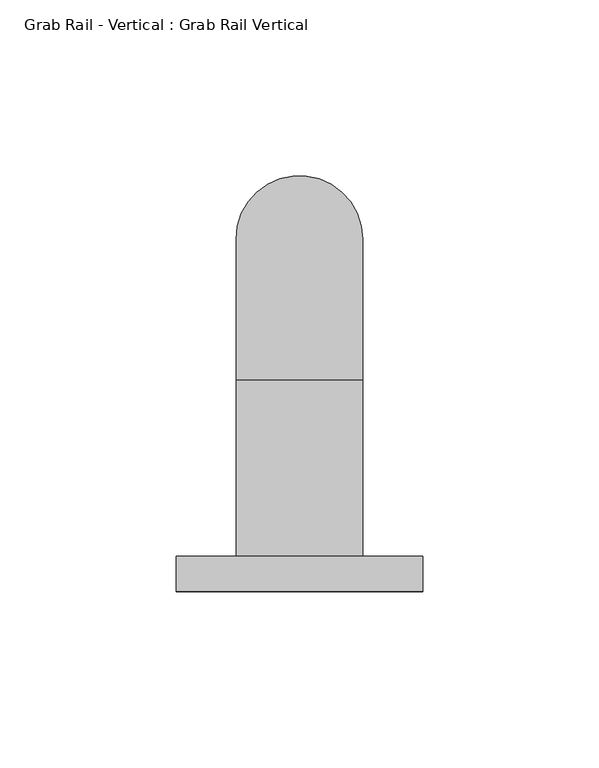
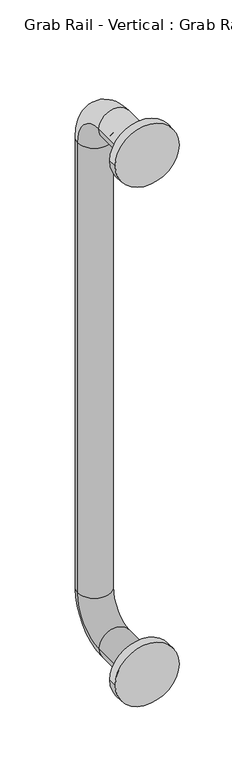
"""IFC4 building model written with IfcOpenShell, lengths in millimetres: flow terminal geometry, Grab Rail - Vertical : Grab Rail Vertical."""

from ifc_helpers import new_model, si_unit, point, frame, frame_2d, origin, place, context, project, spatial, circle_curve, ellipse_curve, trimmed, segment, composite_curve, outline, extrude, source, transform, mapped, element, save
from ifc_brep_helpers import plane_surface, cylinder_surface, revolved_surface, advanced_brep


def grab_rail_vertical_grab_rail_vertical_969059c8(model_context):
    return source(origin(), model_context, "Body", "SolidModel", [
        extrude(outline(composite_curve([segment(trimmed(circle_curve(frame_2d((1400.0, -855.7956665)), 35.0), [point((1400.0, -820.7956665))], [point((1400.0, -890.7956665))], False, "CARTESIAN"), True, "CONTINUOUS"), segment(trimmed(circle_curve(frame_2d((1400.0, -855.7956665)), 35.0), [point((1400.0, -890.7956665))], [point((1400.0, -820.7956665))], False, "CARTESIAN"), True, "CONTINUOUS")], self_intersect=False)), frame((0.0, 0.0, 0.0), z_axis=(0.0, 1.0, 0.0), x_axis=(0.0, 0.0, 1.0)), (0.0, 0.0, 1.0), 10.0),
        extrude(outline(composite_curve([segment(trimmed(circle_curve(frame_2d((800.0, -855.7956665)), 35.0), [point((800.0, -820.7956665))], [point((800.0, -890.7956665))], False, "CARTESIAN"), True, "CONTINUOUS"), segment(trimmed(circle_curve(frame_2d((800.0, -855.7956665)), 35.0), [point((800.0, -890.7956665))], [point((800.0, -820.7956665))], False, "CARTESIAN"), True, "CONTINUOUS")], self_intersect=False)), frame((0.0, 0.0, 0.0), z_axis=(0.0, 1.0, 0.0), x_axis=(0.0, 0.0, 1.0)), (0.0, 0.0, 1.0), 10.0),
        advanced_brep(
        [(-873.7956665, 10.0, 1400.0), (-837.7956665, 10.0, 1400.0), (-873.7956665, 60.0, 1400.0), (-837.7956665, 60.0, 1400.0), (-837.7956665, 100.0, 1360.0), (-873.7956665, 100.0, 1360.0), (-873.7956665, 100.0, 840.0), (-837.7956665, 100.0, 840.0), (-837.7956665, 60.0, 800.0), (-873.7956665, 60.0, 800.0), (-873.7956665, 10.0, 800.0), (-837.7956665, 10.0, 800.0)],
        [
            (0, 1, circle_curve(frame((-855.7956665, 10.0, 1400.0), z_axis=(0.0, -1.0, 0.0), x_axis=(1.0, 0.0, 0.0)), 18.0)),
            (1, 0, circle_curve(frame((-855.7956665, 10.0, 1400.0), z_axis=(0.0, -1.0, 0.0), x_axis=(1.0, 0.0, 0.0)), 18.0)),
            (0, 2),
            (2, 3, circle_curve(frame((-855.7956665, 60.0, 1400.0), z_axis=(0.0, -1.0, 0.0), x_axis=(1.0, 0.0, 0.0)), 18.0)),
            (3, 1),
            (3, 2, circle_curve(frame((-855.7956665, 60.0, 1400.0), z_axis=(0.0, -1.0, 0.0), x_axis=(1.0, 0.0, 0.0)), 18.0)),
            (4, 3, circle_curve(frame((-837.7956665, 60.0, 1360.0), z_axis=(1.0, 0.0, 0.0), x_axis=(0.0, 0.0, 1.0)), 40.0)),
            (2, 5, circle_curve(frame((-873.7956665, 60.0, 1360.0), z_axis=(-1.0, 0.0, 0.0), x_axis=(0.0, 0.0, 1.0)), 40.0)),
            (5, 4, circle_curve(frame((-855.7956665, 100.0, 1360.0), z_axis=(0.0, 0.0, 1.0), x_axis=(1.0, 0.0, 0.0)), 18.0)),
            (4, 5, circle_curve(frame((-855.7956665, 100.0, 1360.0), z_axis=(0.0, 0.0, 1.0), x_axis=(1.0, 0.0, 0.0)), 18.0)),
            (5, 6),
            (6, 7, circle_curve(frame((-855.7956665, 100.0, 840.0), z_axis=(0.0, 0.0, 1.0), x_axis=(1.0, 0.0, 0.0)), 18.0)),
            (7, 4),
            (7, 6, circle_curve(frame((-855.7956665, 100.0, 840.0), z_axis=(0.0, 0.0, 1.0), x_axis=(1.0, 0.0, 0.0)), 18.0)),
            (8, 7, circle_curve(frame((-837.7956665, 60.0, 840.0), z_axis=(1.0, 0.0, 0.0), x_axis=(0.0, 1.0, 0.0)), 40.0)),
            (6, 9, circle_curve(frame((-873.7956665, 60.0, 840.0), z_axis=(-1.0, 0.0, 0.0), x_axis=(0.0, 1.0, 0.0)), 40.0)),
            (9, 8, circle_curve(frame((-855.7956665, 60.0, 800.0), z_axis=(0.0, 1.0, 0.0), x_axis=(1.0, 0.0, 0.0)), 18.0)),
            (8, 9, circle_curve(frame((-855.7956665, 60.0, 800.0), z_axis=(0.0, 1.0, 0.0), x_axis=(1.0, 0.0, 0.0)), 18.0)),
            (10, 11, circle_curve(frame((-855.7956665, 10.0, 800.0), z_axis=(0.0, -1.0, 0.0), x_axis=(1.0, 0.0, 0.0)), 18.0)),
            (11, 10, circle_curve(frame((-855.7956665, 10.0, 800.0), z_axis=(0.0, -1.0, 0.0), x_axis=(1.0, 0.0, 0.0)), 18.0)),
            (9, 10),
            (11, 8),
        ],
        [
            plane_surface(frame((-855.7956665, 10.0, 1400.0), z_axis=(0.0, -1.0, 0.0), x_axis=(1.0, 0.0, 0.0))),
            cylinder_surface(frame((-855.7956665, 10.0, 1400.0), z_axis=(0.0, -1.0, 0.0), x_axis=(1.0, 0.0, 0.0)), 18.0),
            revolved_surface(trimmed(ellipse_curve(frame((-855.7956665, 60.0, 1400.0), z_axis=(0.0, -1.0, 0.0), x_axis=(1.0, 0.0, 0.0)), 18.0, 18.0), [point((-873.7956665, 60.0, 1400.0))], [point((-837.7956665, 60.0, 1400.0))], True, "CARTESIAN"), (-855.7956665, 60.0, 1360.0), (-1.0, 0.0, 0.0)),
            revolved_surface(trimmed(ellipse_curve(frame((-855.7956665, 60.0, 1400.0), z_axis=(0.0, -1.0, 0.0), x_axis=(1.0, 0.0, 0.0)), 18.0, 18.0), [point((-837.7956665, 60.0, 1400.0))], [point((-873.7956665, 60.0, 1400.0))], True, "CARTESIAN"), (-855.7956665, 60.0, 1360.0), (-1.0, 0.0, 0.0)),
            cylinder_surface(frame((-855.7956665, 100.0, 1360.0), z_axis=(0.0, 0.0, 1.0), x_axis=(1.0, 0.0, 0.0)), 18.0),
            revolved_surface(trimmed(ellipse_curve(frame((-855.7956665, 100.0, 840.0), z_axis=(0.0, 0.0, 1.0), x_axis=(1.0, 0.0, 0.0)), 18.0, 18.0), [point((-873.7956665, 100.0, 840.0))], [point((-837.7956665, 100.0, 840.0))], True, "CARTESIAN"), (-855.7956665, 60.0, 840.0), (-1.0, 0.0, 0.0)),
            revolved_surface(trimmed(ellipse_curve(frame((-855.7956665, 100.0, 840.0), z_axis=(0.0, 0.0, 1.0), x_axis=(1.0, 0.0, 0.0)), 18.0, 18.0), [point((-837.7956665, 100.0, 840.0))], [point((-873.7956665, 100.0, 840.0))], True, "CARTESIAN"), (-855.7956665, 60.0, 840.0), (-1.0, 0.0, 0.0)),
            plane_surface(frame((-855.7956665, 10.0, 800.0), z_axis=(0.0, -1.0, 0.0), x_axis=(1.0, 0.0, 0.0))),
            cylinder_surface(frame((-855.7956665, 60.0, 800.0), z_axis=(0.0, 1.0, 0.0), x_axis=(1.0, 0.0, 0.0)), 18.0),
        ],
        [
            (0, [[1, 2]]),
            (1, [[-1, 3, 4, 5]]),
            (1, [[-2, -5, 6, -3]]),
            (2, [[7, -4, 8, 9]]),
            (3, [[-8, -6, -7, 10]]),
            (4, [[-9, 11, 12, 13]]),
            (4, [[-10, -13, 14, -11]]),
            (5, [[15, -12, 16, 17]]),
            (6, [[-16, -14, -15, 18]]),
            (7, [[19, 20]]),
            (8, [[-17, 21, -20, 22]]),
            (8, [[-18, -22, -19, -21]]),
        ],
    ),
    ])


if __name__ == "__main__":
    model = new_model("IFC4")
    model_context = context("Model", 3, world=origin())
    ifc_project = project(units=[si_unit("LENGTHUNIT", "METRE", prefix="MILLI")], contexts=[model_context])
    site = spatial("IfcSite", under=ifc_project)
    building = spatial("IfcBuilding", under=site)
    placement = place(None, origin())
    grab_rail_vertical_grab_rail_vertical_shape = grab_rail_vertical_grab_rail_vertical_969059c8(model_context)
    element("IfcFlowTerminal", 1, ObjectType="Grab Rail - Vertical : Grab Rail Vertical", at=placement, inside=building, context=model_context, shape_type="MappedRepresentation", body=[
        mapped(grab_rail_vertical_grab_rail_vertical_shape, transform((0.0, 0.0, 0.0), x_axis=(1.0, 0.0, 0.0), y_axis=(0.0, 1.0, 0.0), z_axis=(0.0, 0.0, 1.0))),
    ])
    save(model, "model.ifc")

# Revit data of these elements
# Type "Grab Rail - Vertical : Grab Rail Vertical"
#   Keynote = "N13"
#   Material SanitaryWare [instance default] = Metal - White powder coated
#   Default Elevation = 0
#   Assembly Code = ""
# Element 1 (IfcFlowTerminal, "Grab Rail - Vertical : Grab Rail Vertical")
#   Materials on its faces: "Metal - White powder coated"
# Materials
#   "Metal - White powder coated": colour RGB 249 249 249, transparency 0
